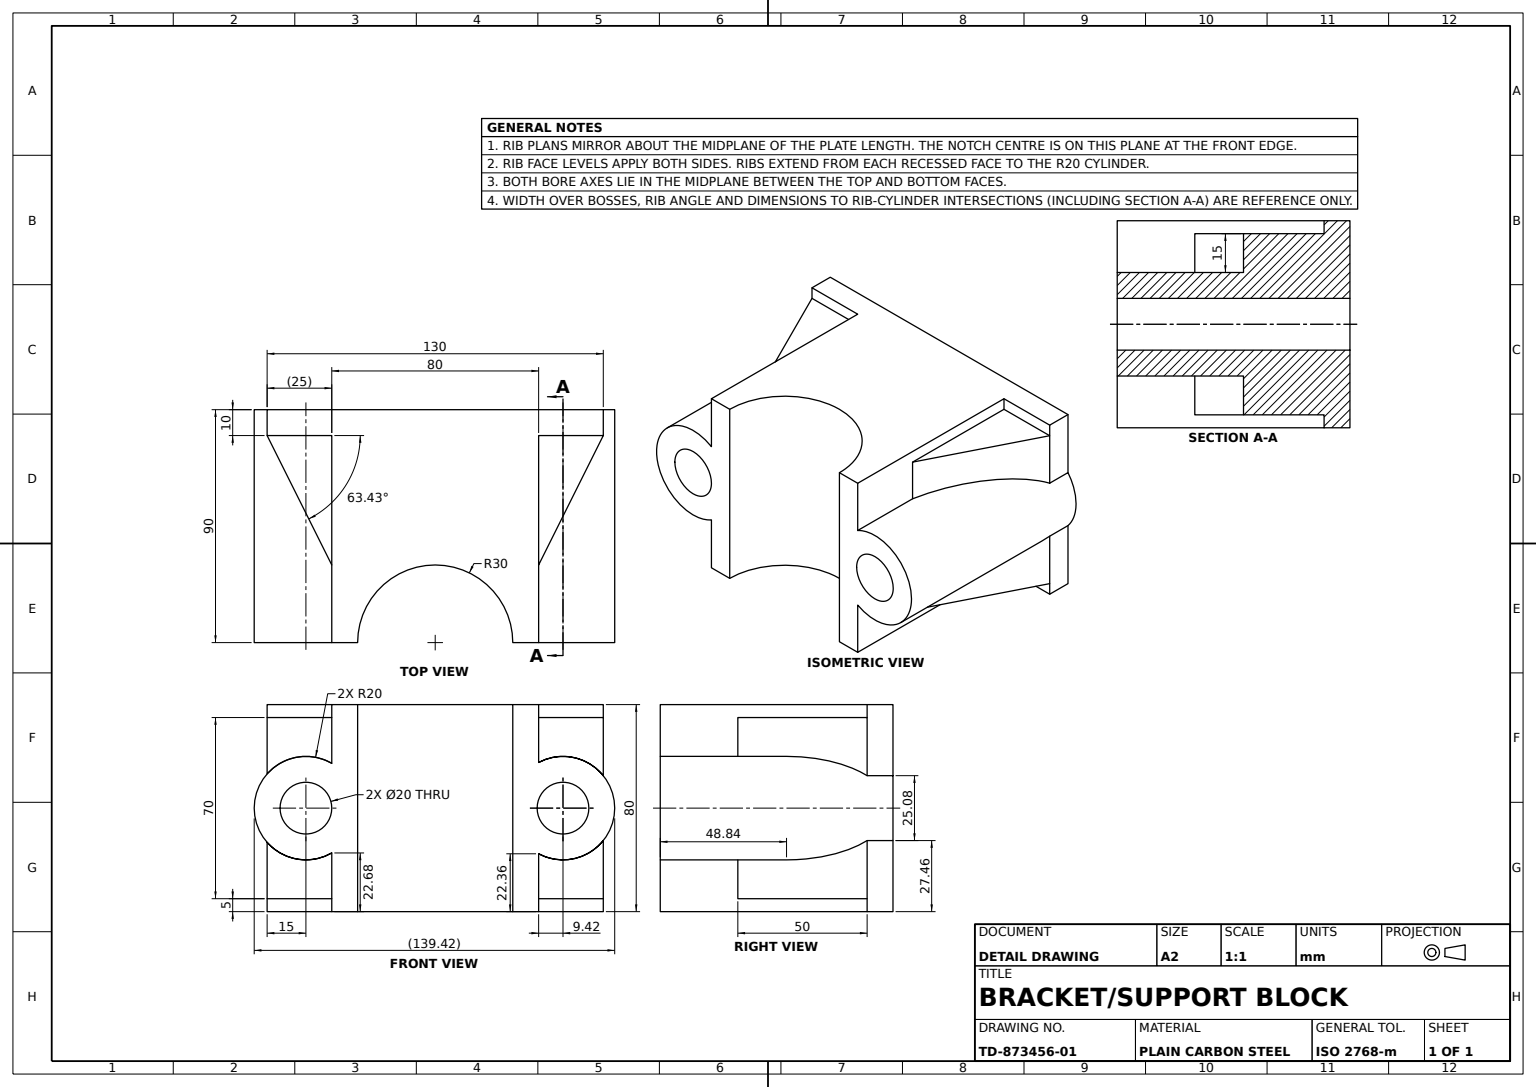
SolidWorks part; units mm, degrees
material "Plain Carbon Steel"
ref_plane "Front Plane" through (0, 0, 0) normal (0, 0, 1) x (1, 0, 0)
ref_plane "Top Plane" through (0, 0, 0) normal (0, 1, 0) x (1, 0, 0)
ref_plane "Right Plane" through (0, 0, 0) normal (1, 0, 0) x (0, 0, -1)
sketch "Base Plate Sketch" plane through (0, 0, 0) normal (0, 0, 1) x (1, 0, 0)
  line L0 (0, 0) -> (130, 0)
  line L1 (130, 0) -> (130, 80)
  line L2 (130, 80) -> (0, 80)
  line L3 (0, 80) -> (0, 0)
  dimension "D1" = 130
  dimension "D2" = 80
extrude "Base Plate 10mm" add sketch "Base Plate Sketch" along normal blind 10
sketch "Main Body Profile" plane through (0, 0, 0) normal (0, -1, 0) x (1, 0, 0)
  line L0 (65, 10) -> (105, 10)
  line L1 (0, 10) -> (130, 10) construction
  line L2 (35, 90) -> (35, 10)
  line L3 (35, 10) -> (95, 10)
  line L4 (95, 10) -> (95, 90)
  line L5 (105, 10) -> (105, 90)
  line L6 (105, 90) -> (95, 90)
  line L7 (65, 10) -> (25, 10)
  line L8 (25, 10) -> (25, 90)
  line L9 (25, 90) -> (35, 90)
  line L10 (130, 10) -> (130, 0) construction
  line L11 (0, 0) -> (130, 0) construction
  arc A0 (35, 90) -> (95, 90) centre (65, 90) ccw
  line M3 (130, 10) -> (0, 10)
  dimension "D1" = 60
  dimension "D2" = 30
  dimension "D3" = 25
  dimension "D4" = 65
  dimension "D5" = 90
extrude "Main Body" add sketch "Main Body Profile" against normal blind 80 contours L9 L8 L2 M3 | A0 L2 L0 L4 M3 | L5 L6 L4 M3
sketch "Side Wall A Sketch" plane through (0, 0, 90) normal (0, 0, 1) x (1, 0, 0)
  line L0 (105, 57.6434) -> (105, 22.3566)
  line L1 (105, 0) -> (95, 0) construction
  line L5 (105, 80) -> (105, 0) construction
  line L6 (105, 80) -> (105, 0) construction
  arc A0 (105, 22.3566) -> (105, 57.6434) centre (114.4186, 40) ccw
  dimension "D1" = 40
  dimension "D2" = 20
  dimension "D3" = 9.4186
  dimension "D4" = 22.3566
extrude "Side Wall A" add sketch "Side Wall A Sketch" against normal blind 90
sketch "Side Wall B Sketch" plane through (0, 0, 90) normal (0, 0, 1) x (1, 0, 0)
  line L0 (35, 80) -> (35, 0) construction
  line L1 (25, 0) -> (35, 0) construction
  line L5 (25, 57.3205) -> (25, 22.6795)
  line L6 (25, 80) -> (25, 0) construction
  line L7 (25, 80) -> (25, 0) construction
  arc A0 (25, 57.3205) -> (25, 22.6795) centre (15, 40) ccw
  dimension "D1" = 40
  dimension "D2" = 20
  dimension "D3" = 20
  dimension "D4" = 22.6795
extrude "Side Wall B" add sketch "Side Wall B Sketch" against normal blind 90
sketch "Half Bore Sketch" plane through (0, 0, 90) normal (0, 0, 1) x (1, 0, 0)
  circle A0 centre (114.4186, 40) radius 10
  circle A1 centre (15, 40) radius 10
  dimension "D1" = 20
  dimension "D2" = 20
  dimension "D3" = 20
extrude "Half Bore Cut" cut sketch "Half Bore Sketch" against normal blind 90
sketch "Rib A Sketch" plane through (0, 0, 0) normal (0, -1, 0) x (1, 0, 0)
  line L0 (105, 10) -> (105, 60)
  line L1 (105, 10) -> (105, 90) construction
  line L2 (105, 60) -> (130, 10)
  line L3 (130, 10) -> (105, 10)
  line L5 (0, 0) -> (130, 0) construction
  dimension "D1" = 60
extrude "Rib A" add sketch "Rib A Sketch" against normal blind 28
sketch "Rib B Sketch" plane through (0, 0, 0) normal (0, -1, 0) x (1, 0, 0)
  line L0 (25, 10) -> (25, 60)
  line L1 (25, 90) -> (25, 10) construction
  line L2 (25, 60) -> (0, 10)
  line L3 (0, 10) -> (25, 10)
  dimension "D1" = 50
extrude "Rib B" add sketch "Rib B Sketch" against normal blind 28
sketch "Boss Sketch" plane through (0, 80, 0) normal (0, 1, 0) x (1, 0, 0)
  line L0 (105, -10) -> (105, -60)
  line L1 (105, -10) -> (105, -90) construction
  line L2 (105, -60) -> (130, -10)
  line L3 (130, -10) -> (105, -10)
  line L4 (25, -10) -> (25, -60)
  line L5 (25, -10) -> (25, -90) construction
  line L6 (25, -60) -> (0, -10)
  line L7 (0, -10) -> (25, -10)
  line L9 (130, 0) -> (0, 0) construction
  dimension "D1" = 60
extrude "Boss" add sketch "Boss Sketch" against normal blind 28
sketch "Recess A Sketch" plane through (0, 0, 0) normal (0, -1, 0) x (1, 0, 0)
  line L0 (25, 60) -> (25, 10)
  line L1 (25, 10) -> (0, 10)
  line L2 (0, 10) -> (25, 60)
  line L3 (105, 60) -> (105, 10)
  line L4 (105, 10) -> (130, 10)
  line L5 (130, 10) -> (105, 60)
extrude "Recess Cut A 5mm" cut sketch "Recess A Sketch" against normal blind 5
sketch "Recess B Sketch" plane through (0, 80, 0) normal (0, 1, 0) x (1, 0, 0)
  line L0 (25, -60) -> (25, -10)
  line L1 (25, -10) -> (0, -10)
  line L2 (0, -10) -> (25, -60)
  line L3 (105, -60) -> (105, -10)
  line L4 (105, -10) -> (130, -10)
  line L5 (130, -10) -> (105, -60)
extrude "Recess Cut B 5mm" cut sketch "Recess B Sketch" against normal blind 5
